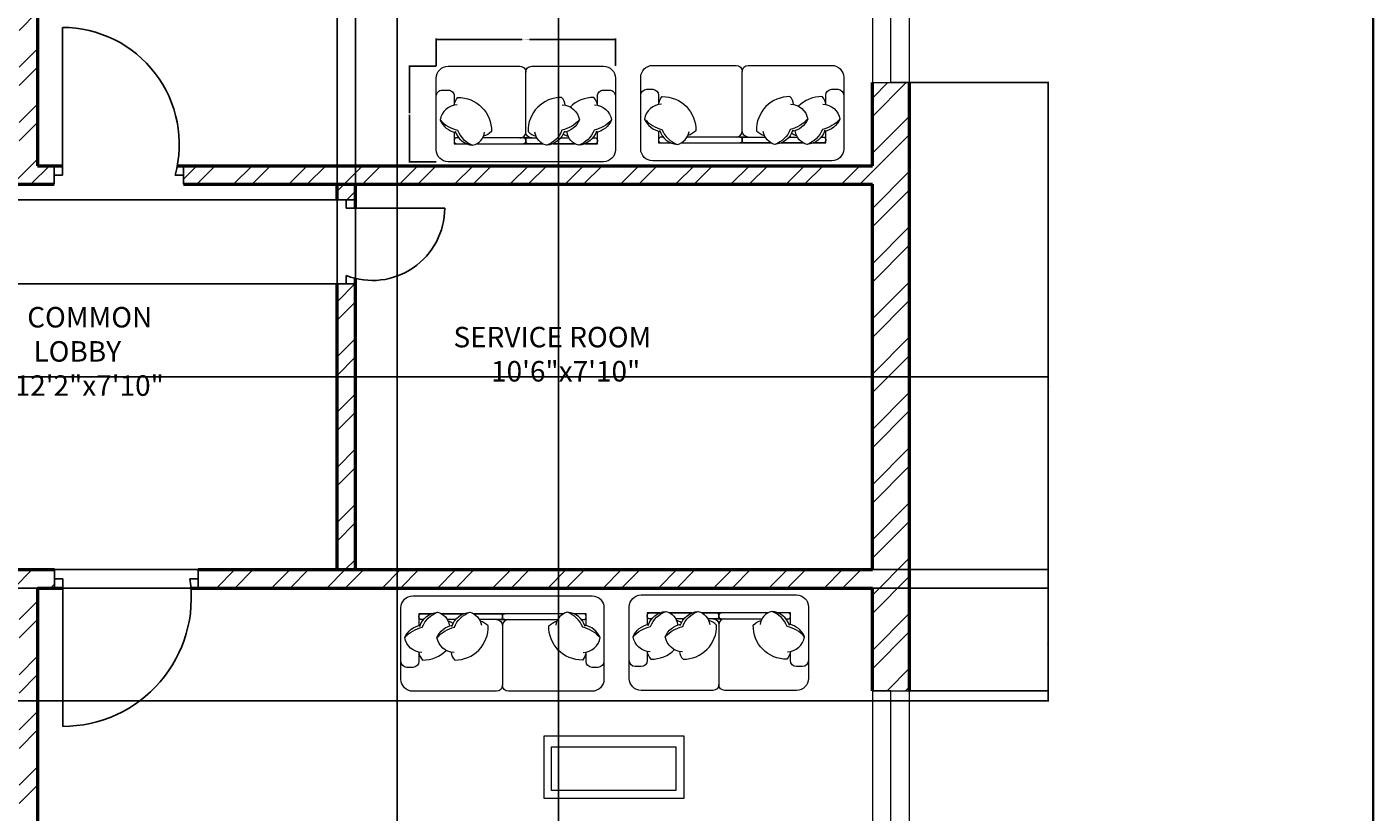
# Model space of a CAD drawing. Units: inches. Extents: x 2310 to 2937, y 1113 to 2410.
# Tile 16 of 23: x 2609 to 2937, y 1940 to 2132. Entities that reach past the tile are written whole.
import ezdxf

# ---------------------------------------------------------------- set-up
doc = ezdxf.new("R2010")
doc.units = ezdxf.units.IN
for name, color, linetype, lineweight in [('A-ANNO-DIMS', 2, 'Continuous', 18), ('A-ANNO-TTLB', 7, 'Continuous', 35), ('A-AREA-IDEN', 7, 'Continuous', 18), ('A-DOOR', 31, 'Continuous', 25), ('A-FURN', 8, 'Continuous', 18), ('A-GLAZ', 191, 'Continuous', 20), ('A-WALL', 7, 'Continuous', 50), ('A-WALL-PATT', 85, 'Continuous', 13)]:
    doc.layers.add(name, color=color, linetype=linetype, lineweight=lineweight)
doc.styles.get("Standard").update_dxf_attribs({"font": 'arial.ttf'})
doc.dimstyles.get("Standard").update_dxf_attribs({"dimtxt": 0.18, "dimasz": 0.18, "dimexe": 0.18, "dimexo": 0.0625, "dimgap": 0.09, "dimtad": 0, "dimtih": 1, "dimtoh": 1, "dimdec": 4, "dimzin": 0, "dimdsep": 46, "dimtxsty": 'Standard', "dimcen": 0.09, "dimadec": 0, "dimazin": 0, "dimtfac": 1, "dimtdec": 4, "dimtofl": 0, "dimtmove": 0, "dimatfit": 3, "dimfxl": 1, "dimtolj": 1, "dimtzin": 0, "dimarcsym": 0})

# ---------------------------------------------------------------- blocks, each defined once
blk = doc.blocks.new('SOFA-COMPACT')
at = {"ltscale": 0.03}
blk.add_lwpolyline([(20.37, 23.28, -0.414214), (21.83, 21.83, -0.414214), (23.28, 23.28), (40.75, 23.28, -0.414214), (43.66, 20.37), (43.66, 2.91, -0.414214), (40.75, 0), (2.91, 0, -0.414214), (0, 2.91), (0, 20.37, -0.414214), (2.91, 23.28), (20.37, 23.28, -0.414214), (21.83, 21.83, -0.414214), (23.28, 23.28)], format="xyb", dxfattribs=at)
for points in [[(20.37, 5.82, 0.414214), (21.83, 7.28), (21.83, 21.83, 0.414214)], [(23.28, 5.82, -0.414214), (21.83, 7.28), (21.83, 21.83, -0.414214)], [(0, 16.01, -0.414214), (1.46, 17.46), (2.91, 17.46, -0.414214), (4.37, 16.01), (4.37, 13.75)], [(39.29, 13.75), (39.29, 16.01, -0.414214), (40.75, 17.46), (42.2, 17.46, -0.414214), (43.66, 16.01)], [(5.1, 13.84, 0.356772), (0.93, 10.17, 0.249542), (4.7, 7.15, -9.61688)], [(4.36, 13.75, -0.165541), (5.26, 15.67, -0.425989), (13.44, 7.34, -0.121523), (11.5, 6.19, 7.115464)], [(31.45, 13.75, 0.165541), (30.55, 15.67, 0.425989), (22.38, 7.34, 0.121523), (24.32, 6.19, -7.115464)], [(30.72, 13.84, -0.356772), (34.89, 10.17, -0.249542), (31.11, 7.15, 9.61688)], [(39.29, 13.75, 0.165541), (38.39, 15.67, 0.200231), (32.62, 13.33, 0.121523)], [(38.56, 13.84, -0.356772), (42.73, 10.17, -0.249542), (38.95, 7.15, 9.61688)], [(0.93, 10.17, 0.14773), (5.18, 7.67, 0.213343), (8.93, 4, 0.178662)], [(34.89, 10.17, -0.14773), (30.64, 7.67, -0.213343), (26.88, 4, -0.178662)], [(42.73, 10.17, -0.14773), (38.48, 7.67, -0.213343), (34.72, 4, -0.178662)], [(4.59, 7.47, 0.306663), (8.93, 4, 0.30633), (11.77, 7.17, -0.872847)], [(20.37, 5.82, 0.414214), (21.83, 7.28)], [(23.28, 5.82, -0.414214), (21.83, 7.28)], [(31.22, 7.47, -0.306663), (26.88, 4, -0.30633), (24.05, 7.17, 0.872847)], [(30.94, 6.76, 0.071865), (32.16, 6.19, -7.115464)], [(39.06, 7.47, -0.306663), (34.72, 4, -0.30633), (31.89, 7.17, 0.872847)], [(36.23, 4.37), (39.29, 4.37), (39.29, 7.23, -0.414214)], [(5.48, 5.82), (4.95, 5.82, 0.414214), (4.37, 5.24), (4.37, 4.95, 0.414214), (4.95, 4.37)], [(4.95, 4.37), (7.43, 4.37, 0.414214)], [(9.85, 4.37), (21.25, 4.37, 0.414214), (21.83, 4.95), (21.83, 5.24, 0.414214), (21.25, 5.82), (11.31, 5.82, 0.414214)], [(25.97, 4.37), (22.41, 4.37, -0.414214), (21.83, 4.95), (21.83, 5.24, -0.414214), (22.41, 5.82), (24.5, 5.82, -0.414214)], [(33.81, 4.37), (28.39, 4.37, -0.414214)], [(30.34, 5.82), (32.34, 5.82, -0.414214)], [(38.71, 4.37), (36.23, 4.37, -0.414214)], [(38.18, 5.82), (38.71, 5.82, -0.414214), (39.29, 5.24), (39.29, 4.95, -0.414214), (38.71, 4.37)]]:
    blk.add_lwpolyline(points, format="xyb")
for points in [[(4.37, 7.23), (4.37, 4.37), (7.43, 4.37)], [(9.85, 4.37), (25.97, 4.37)], [(28.39, 4.37), (33.81, 4.37)]]:
    blk.add_lwpolyline(points)
blk.add_lwpolyline([(21.25, 4.37), (22.41, 4.37, -0.414214), (21.83, 4.95), (21.83, 5.24, -0.414214), (22.41, 5.82), (21.25, 5.82, -0.414214), (21.83, 5.24), (21.83, 4.95, -0.414214)], format="xyb", close=True)
blk = doc.blocks.new('WIN-60IN')
for p, q in [((4.5, 60), (0, 60)), ((0, 60), (9, 60)), ((0, 60), (0, 0)), ((4.5, 0), (4.5, 60)), ((9, 60), (9, 0)), ((0, 0), (9, 0)), ((9, 0), (4.5, 0))]:
    blk.add_line(p, q)
blk = doc.blocks.new('*D37')
at = {"layer": 'A-ANNO-DIMS', "color": 0, "lineweight": -2, "transparency": 16777216}
for p, q in [((2708.68, 2122.37), (2708.68, 2129.03)), ((2708.86, 2128.85), (2729.6, 2128.85)), ((2752.16, 2128.85), (2731.41, 2128.85)), ((2752.34, 2122.37), (2752.34, 2129.03))]:
    blk.add_line(p, q, dxfattribs=at)
at = {"layer": 'A-ANNO-DIMS', "color": 0, "transparency": 16777216}
for points in [[(2708.86, 2128.88), (2708.86, 2128.82), (2708.68, 2128.85)], [(2752.16, 2128.88), (2752.16, 2128.82), (2752.34, 2128.85)]]:
    blk.add_solid(points, dxfattribs=at)
at = {"layer": 'Defpoints', "color": 0, "transparency": 16777216}
for p in [(2752.34, 2128.85), (2708.68, 2122.3), (2752.34, 2122.3)]:
    blk.add_point(p, dxfattribs=at)
at = {"layer": 'A-ANNO-DIMS', "color": 0, "transparency": 16777216, "insert": (2730.51, 2128.85), "char_height": 0.18, "attachment_point": 5}
blk.add_mtext('\\A1;SOFA 44 TYP.', dxfattribs=at)
blk = doc.blocks.new('*D38')
at = {"layer": 'A-ANNO-DIMS', "color": 0, "lineweight": -2, "transparency": 16777216}
for p, q in [((2708.62, 2122.3), (2701.95, 2122.3)), ((2702.13, 2122.12), (2702.13, 2110.84)), ((2702.13, 2099.2), (2702.13, 2110.48)), ((2708.62, 2099.02), (2701.95, 2099.02))]:
    blk.add_line(p, q, dxfattribs=at)
at = {"layer": 'A-ANNO-DIMS', "color": 0, "transparency": 16777216}
for points in [[(2702.1, 2122.12), (2702.16, 2122.12), (2702.13, 2122.3)], [(2702.1, 2099.2), (2702.16, 2099.2), (2702.13, 2099.02)]]:
    blk.add_solid(points, dxfattribs=at)
at = {"layer": 'Defpoints', "color": 0, "transparency": 16777216}
for p in [(2702.13, 2122.3), (2708.68, 2122.3), (2708.68, 2099.02)]:
    blk.add_point(p, dxfattribs=at)
at = {"layer": 'A-ANNO-DIMS', "color": 0, "transparency": 16777216, "insert": (2702.13, 2110.66), "char_height": 0.18, "attachment_point": 5}
blk.add_mtext('\\A1;23 TYP.', dxfattribs=at)
blk = doc.blocks.new('*D42')
at = {"layer": 'A-ANNO-DIMS', "color": 0, "lineweight": -2, "transparency": 16777216}
for p, q in [((2699.14, 2347.45), (2699.14, 1649.5)), ((2738.49, 2347.45), (2738.49, 1649.5)), ((2699.32, 1649.68), (2718.42, 1649.68)), ((2738.31, 1649.68), (2719.21, 1649.68))]:
    blk.add_line(p, q, dxfattribs=at)
at = {"layer": 'A-ANNO-DIMS', "color": 0, "transparency": 16777216}
for points in [[(2699.32, 1649.71), (2699.32, 1649.65), (2699.14, 1649.68)], [(2738.31, 1649.71), (2738.31, 1649.65), (2738.49, 1649.68)]]:
    blk.add_solid(points, dxfattribs=at)
at = {"layer": 'Defpoints', "color": 0, "transparency": 16777216}
for p in [(2699.14, 2347.51), (2738.49, 2347.51), (2738.49, 1649.68)]:
    blk.add_point(p, dxfattribs=at)
at = {"layer": 'A-ANNO-DIMS', "color": 0, "transparency": 16777216, "insert": (2718.81, 1649.68), "char_height": 0.18, "attachment_point": 5}
blk.add_mtext('\\A1;39.35', dxfattribs=at)
blk = doc.blocks.new('*D48')
at = {"layer": 'A-ANNO-DIMS', "color": 0, "lineweight": -2, "transparency": 16777216}
for p, q in [((2824.05, 2118.3), (2858.02, 2118.3)), ((2857.84, 2118.12), (2857.84, 2044.32)), ((2857.84, 1970.16), (2857.84, 2043.96)), ((2824.05, 1969.98), (2858.02, 1969.98))]:
    blk.add_line(p, q, dxfattribs=at)
at = {"layer": 'A-ANNO-DIMS', "color": 0, "transparency": 16777216}
for points in [[(2857.81, 2118.12), (2857.87, 2118.12), (2857.84, 2118.3)], [(2857.81, 1970.16), (2857.87, 1970.16), (2857.84, 1969.98)]]:
    blk.add_solid(points, dxfattribs=at)
at = {"layer": 'Defpoints', "color": 0, "transparency": 16777216}
for p in [(2823.99, 2118.3), (2857.84, 2118.3), (2823.99, 1969.98)]:
    blk.add_point(p, dxfattribs=at)
at = {"layer": 'A-ANNO-DIMS', "color": 0, "transparency": 16777216, "insert": (2857.84, 2044.14), "char_height": 0.18, "attachment_point": 5}
blk.add_mtext('\\A1;148.32', dxfattribs=at)
blk = doc.blocks.new('*D57')
at = {"layer": 'A-ANNO-DIMS', "color": 0, "lineweight": -2, "transparency": 16777216}
for p, q in [((2403.55, 1995.01), (2858.02, 1995.01)), ((2857.84, 1994.83), (2857.84, 1981.45)), ((2857.84, 1967.7), (2857.84, 1981.09)), ((2403.55, 1967.52), (2858.02, 1967.52))]:
    blk.add_line(p, q, dxfattribs=at)
at = {"layer": 'A-ANNO-DIMS', "color": 0, "transparency": 16777216}
for points in [[(2857.81, 1994.83), (2857.87, 1994.83), (2857.84, 1995.01)], [(2857.81, 1967.7), (2857.87, 1967.7), (2857.84, 1967.52)]]:
    blk.add_solid(points, dxfattribs=at)
at = {"layer": 'Defpoints', "color": 0, "transparency": 16777216}
for p in [(2403.49, 1995.01), (2403.49, 1967.52), (2857.84, 1967.52)]:
    blk.add_point(p, dxfattribs=at)
at = {"layer": 'A-ANNO-DIMS', "color": 0, "transparency": 16777216, "insert": (2857.84, 1981.27), "char_height": 0.18, "attachment_point": 5}
blk.add_mtext('\\A1;27.49', dxfattribs=at)
blk = doc.blocks.new('*D64')
at = {"layer": 'A-ANNO-DIMS', "color": 0, "lineweight": -2, "transparency": 16777216}
for p, q in [((2524.527191, 2046.513944), (2858.015941, 2046.513944)), ((2857.835941, 2046.333944), (2857.835941, 2023.193944)), ((2857.835941, 1999.693944), (2857.835941, 2022.833944)), ((2524.527191, 1999.513944), (2858.015941, 1999.513944))]:
    blk.add_line(p, q, dxfattribs=at)
at = {"layer": 'A-ANNO-DIMS', "color": 0, "transparency": 16777216}
for points in [[(2857.805941, 2046.333944), (2857.865941, 2046.333944), (2857.835941, 2046.513944)], [(2857.805941, 1999.693944), (2857.865941, 1999.693944), (2857.835941, 1999.513944)]]:
    blk.add_solid(points, dxfattribs=at)
at = {"layer": 'Defpoints', "color": 0, "transparency": 16777216}
for p in [(2524.464691, 2046.513944), (2857.835941, 2046.513944), (2524.464691, 1999.513944)]:
    blk.add_point(p, dxfattribs=at)
at = {"layer": 'A-ANNO-DIMS', "color": 0, "transparency": 16777216, "insert": (2857.835941, 2023.013944), "char_height": 0.18, "attachment_point": 5}
blk.add_mtext('\\A1;47', dxfattribs=at)
blk = doc.blocks.new('*D67')
at = {"layer": 'A-ANNO-DIMS', "color": 0, "lineweight": -2, "transparency": 16777216}
for p, q in [((2684.42, 2089.69), (2360.46, 2089.69)), ((2360.64, 2089.51), (2360.64, 2079.64)), ((2360.64, 2069.41), (2360.64, 2079.28)), ((2684.42, 2069.23), (2360.46, 2069.23))]:
    blk.add_line(p, q, dxfattribs=at)
at = {"layer": 'A-ANNO-DIMS', "color": 0, "transparency": 16777216}
for points in [[(2360.61, 2089.51), (2360.67, 2089.51), (2360.64, 2089.69)], [(2360.61, 2069.41), (2360.67, 2069.41), (2360.64, 2069.23)]]:
    blk.add_solid(points, dxfattribs=at)
at = {"layer": 'Defpoints', "color": 0, "transparency": 16777216}
for p in [(2360.64, 2089.69), (2684.49, 2089.69), (2684.49, 2069.23)]:
    blk.add_point(p, dxfattribs=at)
at = {"layer": 'A-ANNO-DIMS', "color": 0, "transparency": 16777216, "insert": (2360.64, 2079.46), "char_height": 0.18, "attachment_point": 5}
blk.add_mtext('\\A1;20.46', dxfattribs=at)
blk = doc.blocks.new('*D68')
at = {"layer": 'A-ANNO-DIMS', "color": 0, "lineweight": -2, "transparency": 16777216}
for p, q in [((2684.49, 1999.58), (2684.49, 2390.54)), ((2684.67, 2390.36), (2686.48, 2390.36)), ((2688.81, 2390.36), (2686.99, 2390.36)), ((2688.99, 1999.58), (2688.99, 2390.54))]:
    blk.add_line(p, q, dxfattribs=at)
at = {"layer": 'A-ANNO-DIMS', "color": 0, "transparency": 16777216}
for points in [[(2684.67, 2390.39), (2684.67, 2390.33), (2684.49, 2390.36)], [(2688.81, 2390.39), (2688.81, 2390.33), (2688.99, 2390.36)]]:
    blk.add_solid(points, dxfattribs=at)
at = {"layer": 'Defpoints', "color": 0, "transparency": 16777216}
for p in [(2688.99, 2390.36), (2684.49, 1999.51), (2688.99, 1999.51)]:
    blk.add_point(p, dxfattribs=at)
at = {"layer": 'A-ANNO-DIMS', "color": 0, "transparency": 16777216, "insert": (2686.74, 2390.36), "char_height": 0.18, "attachment_point": 5}
blk.add_mtext('\\A1;4.5', dxfattribs=at)

msp = doc.modelspace()

# ---------------------------------------------------------------- hatches: boundary and pattern name
at = {"layer": 'A-WALL-PATT'}
h = msp.add_hatch(dxfattribs=at)
h.set_pattern_fill('ANSI32', color=256)
h.paths.add_polyline_path([(2639.1394, 2356.5139), (2563.662, 2356.5139), (2563.662, 2347.5139), (2606.9859, 2347.5139), (2606.9859, 2210.5139), (2514.2692, 2210.5139), (2514.2692, 2206.0139), (2606.9859, 2206.0139), (2606.9859, 2098.0139), (2602.689, 2098.0139), (2602.689, 2093.5139), (2615.5262, 2093.5139), (2615.5262, 2095.7639), (2615.5262, 2098.0139), (2611.4859, 2098.0139), (2611.4859, 2206.0139), (2703.9391, 2206.0139), (2703.9391, 2208.2639), (2703.9391, 2210.5139), (2611.4859, 2210.5139), (2611.4859, 2347.5139), (2639.1394, 2347.5139)])
h.paths.add_polyline_path([(2823.9859, 2356.5139), (2699.1394, 2356.5139), (2699.1394, 2347.5139), (2738.4859, 2347.5139), (2738.4859, 2343.9266), (2742.9859, 2343.9266), (2742.9859, 2347.5139), (2814.9859, 2347.5139), (2814.9859, 2336.76), (2823.9859, 2336.76)])
h.paths.add_polyline_path([(2823.9859, 2312.76), (2814.9859, 2312.76), (2814.9859, 2299.5139), (2742.9859, 2299.5139), (2742.9859, 2323.0159), (2740.7359, 2323.0159), (2738.4859, 2323.0159), (2738.4859, 2210.5139), (2734.5483, 2210.5139), (2734.5483, 2206.0139), (2746.8769, 2206.0139), (2746.8769, 2208.2639), (2746.8769, 2210.5139), (2742.9859, 2210.5139), (2742.9859, 2295.0139), (2814.9859, 2295.0139), (2814.9859, 2269.8977), (2823.9859, 2269.8977)])
h.paths.add_polyline_path([(2823.9859, 2210.5139), (2823.9859, 2233.8977), (2819.4859, 2233.8977), (2814.9859, 2233.8977), (2814.9859, 2210.5139), (2769.9745, 2210.5139), (2769.9745, 2206.0139), (2814.9859, 2206.0139), (2814.9859, 2178.3027), (2823.9859, 2178.3027)])
h.paths.add_polyline_path([(2823.9859, 2118.3027), (2819.4859, 2118.3027), (2814.9859, 2118.3027), (2814.9859, 2098.0139), (2647.0333, 2098.0139), (2647.0333, 2093.5139), (2814.9859, 2093.5139), (2814.9859, 1999.5139), (2650.6052, 1999.5139), (2650.6052, 1995.0139), (2814.9859, 1995.0139), (2814.9859, 1969.9784), (2823.9859, 1969.9784)])
h.paths.add_polyline_path([(2403.4859, 2093.5139), (2569.9888, 2093.5139), (2569.9888, 2095.7639), (2569.9888, 2098.0139), (2403.4859, 2098.0139), (2403.4859, 2131.7587), (2394.4859, 2131.7587), (2394.4859, 1967.522), (2403.4859, 1967.522), (2403.4859, 1995.0139), (2569.8903, 1995.0139), (2569.8903, 1997.2639), (2569.8903, 1999.5139), (2403.4859, 1999.5139)])
h.paths.add_polyline_path([(2503.662, 2356.5139), (2394.4859, 2356.5139), (2394.4859, 2337.9231), (2398.9859, 2337.9231), (2403.4859, 2337.9231), (2403.4859, 2347.5139), (2475.4859, 2347.5139), (2475.4859, 2343.0384), (2479.9859, 2343.0384), (2479.9859, 2347.5139), (2503.662, 2347.5139)])
h.paths.add_polyline_path([(2498.3065, 1745.5139), (2479.9859, 1745.5139), (2479.9859, 1749.1663), (2477.7359, 1749.1663), (2475.4859, 1749.1663), (2475.4859, 1745.5139), (2403.4859, 1745.5139), (2403.4859, 1753.6409), (2398.9859, 1753.6409), (2394.4859, 1753.6409), (2394.4859, 1736.5139), (2498.3065, 1736.5139), (2498.3065, 1741.0139)])
h.paths.add_polyline_path([(2479.9859, 1882.5139), (2483.9367, 1882.5139), (2483.9367, 1887.0139), (2471.5501, 1887.0139), (2471.5501, 1885.1969), (2471.5501, 1882.5139), (2475.4859, 1882.5139), (2475.4859, 1798.0139), (2403.4859, 1798.0139), (2403.4859, 1828.0433), (2402.2852, 1828.0433), (2394.4859, 1828.0433), (2394.4859, 1777.6409), (2403.4859, 1777.6409), (2403.4859, 1793.5139), (2475.4859, 1793.5139), (2475.4859, 1769.1696), (2479.9859, 1769.1696)])
h.paths.add_polyline_path([(2403.4859, 1907.522), (2398.9859, 1907.522), (2394.4859, 1907.522), (2394.4859, 1864.0433), (2403.4859, 1864.0433), (2403.4859, 1882.5139), (2448.9325, 1882.5139), (2448.9325, 1884.7639), (2448.9325, 1887.0139), (2403.4859, 1887.0139)])
h.paths.add_polyline_path([(2702.2061, 1887.0139), (2611.4859, 1887.0139), (2611.4859, 1995.0139), (2615.6132, 1995.0139), (2615.6132, 1999.5139), (2602.4798, 1999.5139), (2602.4798, 1997.2639), (2602.4798, 1995.0139), (2606.9859, 1995.0139), (2606.9859, 1887.0139), (2516.2443, 1887.0139), (2516.2443, 1884.7639), (2516.2443, 1882.5139), (2606.9859, 1882.5139), (2606.9859, 1745.5139), (2558.3065, 1745.5139), (2558.3065, 1736.5139), (2638.8921, 1736.5139), (2638.8921, 1741.0139), (2638.8921, 1745.5139), (2611.4859, 1745.5139), (2611.4859, 1882.5139), (2702.2061, 1882.5139)])
h.paths.add_polyline_path([(2823.9859, 1909.9784), (2819.4859, 1909.9784), (2814.9859, 1909.9784), (2814.9859, 1887.0139), (2769.144, 1887.0139), (2769.144, 1884.7639), (2769.144, 1882.5139), (2814.9859, 1882.5139), (2814.9859, 1854.1704), (2823.9859, 1854.1704)])
h.paths.add_polyline_path([(2823.9859, 1818.1704), (2819.4859, 1818.1704), (2814.9859, 1818.1704), (2814.9859, 1798.0139), (2742.9859, 1798.0139), (2742.9859, 1882.5139), (2746.805, 1882.5139), (2746.805, 1887.0139), (2733.7334, 1887.0139), (2733.7334, 1884.7639), (2733.7334, 1882.5139), (2738.4859, 1882.5139), (2738.4859, 1771.1728), (2740.7359, 1771.1728), (2742.9859, 1771.1728), (2742.9859, 1793.5139), (2814.9859, 1793.5139), (2814.9859, 1783.6684), (2823.9859, 1783.6684)])
h.paths.add_polyline_path([(2823.9859, 1759.6684), (2814.9859, 1759.6684), (2814.9859, 1745.5139), (2742.9859, 1745.5139), (2742.9859, 1748.9831), (2740.7359, 1748.9831), (2738.4859, 1748.9831), (2738.4859, 1745.5139), (2698.8921, 1745.5139), (2698.8921, 1736.5139), (2823.9859, 1736.5139)])
h = msp.add_hatch(dxfattribs=at)
h.set_pattern_fill('ANSI32', color=256)
h.paths.add_polyline_path([(2688.9859, 2069.228), (2686.7359, 2069.228), (2684.4859, 2069.228), (2684.4859, 1999.5139), (2688.9859, 1999.5139)])
h.paths.add_polyline_path([(2688.9859, 2093.5139), (2684.4859, 2093.5139), (2684.4859, 2089.6861), (2688.9859, 2089.6861)])

# ---------------------------------------------------------------- linework, layer by layer
at = {"layer": 'A-ANNO-TTLB'}
msp.add_lwpolyline([(2310.2498, 2409.8427), (2937.0534, 2409.8427), (2937.0534, 1616.036), (2310.2498, 1616.036)], close=True, dxfattribs=at)
at = {"layer": 'A-DOOR'}
for p, q in [((2617.5262, 2095.7639), (2617.5262, 2131.7639)), ((2615.5262, 2098.0139), (2615.5262, 2093.5139)), ((2647.0333, 2098.0139), (2647.0333, 2093.5139)), ((2615.5262, 2093.5139), (2615.5262, 2095.7639)), ((2615.5262, 2095.7639), (2617.5262, 2095.7639)), ((2647.0333, 2095.7639), (2645.0333, 2095.7639)), ((2647.0333, 2093.5139), (2647.0333, 2095.7639)), ((2684.4859, 2089.6861), (2688.9859, 2089.6861)), ((2688.9859, 2089.6861), (2686.7359, 2089.6861)), ((2686.7359, 2089.6861), (2686.7359, 2087.6861)), ((2686.7359, 2087.6861), (2710.7359, 2087.6861)), ((2686.7359, 2069.228), (2686.7359, 2071.228)), ((2684.4859, 2069.228), (2688.9859, 2069.228)), ((2688.9859, 2069.228), (2686.7359, 2069.228)), ((2615.6132, 1995.0139), (2615.6132, 1999.5139)), ((2615.6132, 1999.5139), (2615.6132, 1997.2639)), ((2650.6052, 1999.5139), (2650.6052, 1999.5139)), ((2650.6052, 1999.5139), (2650.6052, 1995.0139)), ((2615.6132, 1997.2639), (2617.6132, 1997.2639)), ((2617.6132, 1997.2639), (2617.6132, 1961.2639)), ((2650.6052, 1997.2639), (2648.6052, 1997.2639)), ((2650.6052, 1995.0139), (2650.6052, 1997.2639)), ((2650.6052, 1997.2639), (2650.6052, 1997.2639))]:
    msp.add_line(p, q, dxfattribs=at)
for centre, radius, start, end in [((2617.5262, 2103.2551), 28.5089, 344.765874, 90), ((2693.0928, 2087.6861), 17.6431, 248.881039, 0), ((2617.6132, 1992.6044), 31.3404, 270, 8.550242)]:
    msp.add_arc(centre, radius, start, end, dxfattribs=at)
at = {"layer": 'A-FURN', "ltscale": 0.03}
for points in [[(2781.8049, 2122.4997, -0.41421356), (2783.26, 2121.0445, -0.41421356), (2784.7152, 2122.4997), (2805.0879, 2122.4997, -0.41421356), (2807.9983, 2119.5893), (2807.9983, 2102.1271, -0.41421356), (2805.0879, 2099.2167), (2761.4322, 2099.2167, -0.41421356), (2758.5218, 2102.1271), (2758.5218, 2119.5893, -0.41421356), (2761.4322, 2122.4997), (2781.8049, 2122.4997, -0.41421356), (2783.26, 2121.0445, -0.41421356), (2784.7152, 2122.4997)], [(2726.2708, 1969.8431, -0.41421356), (2724.8156, 1971.2983, -0.41421356), (2723.3604, 1969.8431), (2702.9878, 1969.8431, -0.41421356), (2700.0774, 1972.7535), (2700.0774, 1990.2158, -0.41421356), (2702.9878, 1993.1262), (2746.6434, 1993.1262, -0.41421356), (2749.5538, 1990.2158), (2749.5538, 1972.7535, -0.41421356), (2746.6434, 1969.8431), (2726.2708, 1969.8431, -0.41421356), (2724.8156, 1971.2983, -0.41421356), (2723.3604, 1969.8431)], [(2779.0221, 1970.0386, -0.41421356), (2777.5669, 1971.4938, -0.41421356), (2776.1118, 1970.0386), (2758.6495, 1970.0386, -0.41421356), (2755.7391, 1972.949), (2755.7391, 1990.4113, -0.41421356), (2758.6495, 1993.3217), (2796.4844, 1993.3217, -0.41421356), (2799.3948, 1990.4113), (2799.3948, 1972.949, -0.41421356), (2796.4844, 1970.0386), (2779.0221, 1970.0386, -0.41421356), (2777.5669, 1971.4938, -0.41421356), (2776.1118, 1970.0386)]]:
    msp.add_lwpolyline(points, format="xyb", dxfattribs=at)
at = {"layer": 'A-FURN'}
for points in [[(2781.8049, 2105.0374, 0.41421356), (2783.26, 2106.4926), (2783.26, 2121.0445, 0.41421356)], [(2784.7152, 2105.0374, -0.41421356), (2783.26, 2106.4926), (2783.26, 2121.0445, -0.41421356)], [(2758.5218, 2115.2238, -0.41421356), (2759.977, 2116.679), (2761.4322, 2116.679, -0.41421356), (2762.8874, 2115.2238), (2762.8874, 2112.9691)], [(2803.6327, 2112.9691), (2803.6327, 2115.2238, -0.41421356), (2805.0879, 2116.679), (2806.5431, 2116.679, -0.41421356), (2807.9983, 2115.2238)], [(2762.8842, 2112.9685, -0.16554063), (2763.7845, 2114.8912, -0.42598917), (2771.9571, 2106.5549, -0.12152332), (2770.0171, 2105.4059, 7.11546429)], [(2795.7968, 2112.9685, 0.16554063), (2794.8966, 2114.8912, 0.42598917), (2786.724, 2106.5549, 0.12152332), (2788.664, 2105.4059, -7.11546429)], [(2803.6359, 2112.9685, 0.16554063), (2802.7356, 2114.8912, 0.20023115), (2796.9591, 2112.5495, 0.12152332)], [(2763.6177, 2113.0572, 0.35677236), (2759.448, 2109.3892, 0.24954205), (2763.2261, 2106.3665, -9.61688035)], [(2795.0634, 2113.0572, -0.35677236), (2799.2331, 2109.3892, -0.24954205), (2795.4549, 2106.3665, 9.61688035)], [(2802.9024, 2113.0572, -0.35677236), (2807.0721, 2109.3892, -0.24954205), (2803.294, 2106.3665, 9.61688035)], [(2759.448, 2109.3892, 0.14772988), (2763.7011, 2106.8884, 0.21334276), (2767.4538, 2103.2204, 0.17866181)], [(2799.2331, 2109.3892, -0.14772988), (2794.98, 2106.8884, -0.21334276), (2791.2272, 2103.2204, -0.17866181)], [(2807.0721, 2109.3892, -0.14772988), (2802.819, 2106.8884, -0.21334276), (2799.0663, 2103.2204, -0.17866181)], [(2763.9979, 2105.0374), (2763.4695, 2105.0374, 0.41421356), (2762.8874, 2104.4554), (2762.8874, 2104.1643, 0.41421356), (2763.4695, 2103.5823)], [(2763.1135, 2106.689, 0.30666349), (2767.4538, 2103.2204, 0.30632997), (2770.2892, 2106.3882, -0.87284716)], [(2763.4695, 2103.5823), (2765.9487, 2103.5823, 0.41421356)], [(2768.3696, 2103.5823), (2782.678, 2103.5823, 0.41421356), (2783.26, 2104.1643), (2783.26, 2104.4554, 0.41421356), (2782.678, 2105.0374), (2769.8349, 2105.0374, 0.41421356)], [(2781.8049, 2105.0374, 0.41421356), (2783.26, 2106.4926)], [(2784.7152, 2105.0374, -0.41421356), (2783.26, 2106.4926)], [(2790.3114, 2103.5823), (2783.8421, 2103.5823, -0.41421356), (2783.26, 2104.1643), (2783.26, 2104.4554, -0.41421356), (2783.8421, 2105.0374), (2788.8461, 2105.0374, -0.41421356)], [(2795.5675, 2106.689, -0.30666349), (2791.2272, 2103.2204, -0.30632997), (2788.3918, 2106.3882, 0.87284716)], [(2798.1505, 2103.5823), (2792.7323, 2103.5823, -0.41421356)], [(2794.6832, 2105.0374), (2796.6852, 2105.0374, -0.41421356)], [(2795.283, 2105.9748, 0.07186538), (2796.503, 2105.4059, -7.11546429)], [(2803.4066, 2106.689, -0.30666349), (2799.0663, 2103.2204, -0.30632997), (2796.2309, 2106.3882, 0.87284716)], [(2800.5714, 2103.5823), (2803.6327, 2103.5823), (2803.6327, 2106.442, -0.41421356)], [(2803.0506, 2103.5823), (2800.5714, 2103.5823, -0.41421356)], [(2802.5222, 2105.0374), (2803.0506, 2105.0374, -0.41421356), (2803.6327, 2104.4554), (2803.6327, 2104.1643, -0.41421356), (2803.0506, 2103.5823)], [(2701.0035, 1982.9536, -0.14772988), (2705.2566, 1985.4545, -0.21334276), (2709.0094, 1989.1225, -0.17866181)], [(2707.5043, 1988.7606), (2704.443, 1988.7606), (2704.443, 1985.9008, -0.41421356)], [(2705.5534, 1987.3054), (2705.025, 1987.3054, -0.41421356), (2704.443, 1987.8875), (2704.443, 1988.1785, -0.41421356), (2705.025, 1988.7606)], [(2704.6691, 1985.6538, -0.30666349), (2709.0094, 1989.1225, -0.30632997), (2711.8448, 1985.9547, 0.87284716)], [(2705.025, 1988.7606), (2707.5043, 1988.7606, -0.41421356)], [(2708.8426, 1982.9536, -0.14772988), (2713.0957, 1985.4545, -0.21334276), (2716.8484, 1989.1225, -0.17866181)], [(2709.9252, 1988.7606), (2715.3433, 1988.7606, -0.41421356)], [(2712.5081, 1985.6538, -0.30666349), (2716.8484, 1989.1225, -0.30632997), (2719.6838, 1985.9547, 0.87284716)], [(2717.7642, 1988.7606), (2724.2335, 1988.7606, -0.41421356), (2724.8156, 1988.1785), (2724.8156, 1987.8875, -0.41421356), (2724.2335, 1987.3054), (2719.2295, 1987.3054, -0.41421356)], [(2739.706, 1988.7606), (2725.3977, 1988.7606, 0.41421356), (2724.8156, 1988.1785), (2724.8156, 1987.8875, 0.41421356), (2725.3977, 1987.3054), (2738.2407, 1987.3054, 0.41421356)], [(2744.9622, 1985.6538, 0.30666349), (2740.6218, 1989.1225, 0.30632997), (2737.7864, 1985.9547, -0.87284716)], [(2748.6277, 1982.9536, 0.14772988), (2744.3746, 1985.4545, 0.21334276), (2740.6218, 1989.1225, 0.17866181)], [(2744.6062, 1988.7606), (2742.1269, 1988.7606, 0.41421356)], [(2744.0778, 1987.3054), (2744.6062, 1987.3054, 0.41421356), (2745.1882, 1987.8875), (2745.1882, 1988.1785, 0.41421356), (2744.6062, 1988.7606)], [(2756.6652, 1983.1491, -0.14772988), (2760.9183, 1985.65, -0.21334276), (2764.6711, 1989.318, -0.17866181)], [(2763.166, 1988.9561), (2760.1047, 1988.9561), (2760.1047, 1986.0963, -0.41421356)], [(2761.2152, 1987.5009), (2760.6868, 1987.5009, -0.41421356), (2760.1047, 1988.083), (2760.1047, 1988.374, -0.41421356), (2760.6868, 1988.9561)], [(2760.3308, 1985.8493, -0.30666349), (2764.6711, 1989.318, -0.30632997), (2767.5065, 1986.1502, 0.87284716)], [(2760.6868, 1988.9561), (2763.166, 1988.9561, -0.41421356)], [(2764.5043, 1983.1491, -0.14772988), (2768.7574, 1985.65, -0.21334276), (2772.5101, 1989.318, -0.17866181)], [(2765.5869, 1988.9561), (2771.005, 1988.9561, -0.41421356)], [(2768.1698, 1985.8493, -0.30666349), (2772.5101, 1989.318, -0.30632997), (2775.3455, 1986.1502, 0.87284716)], [(2773.4259, 1988.9561), (2776.9849, 1988.9561, -0.41421356), (2777.5669, 1988.374), (2777.5669, 1988.083, -0.41421356), (2776.9849, 1987.5009), (2774.8912, 1987.5009, -0.41421356)], [(2789.547, 1988.9561), (2778.149, 1988.9561, 0.41421356), (2777.5669, 1988.374), (2777.5669, 1988.083, 0.41421356), (2778.149, 1987.5009), (2788.0817, 1987.5009, 0.41421356)], [(2794.8031, 1985.8493, 0.30666349), (2790.4628, 1989.318, 0.30632997), (2787.6274, 1986.1502, -0.87284716)], [(2798.4686, 1983.1491, 0.14772988), (2794.2155, 1985.65, 0.21334276), (2790.4628, 1989.318, 0.17866181)], [(2794.4471, 1988.9561), (2791.9679, 1988.9561, 0.41421356)], [(2793.9187, 1987.5009), (2794.4471, 1987.5009, 0.41421356), (2795.0292, 1988.083), (2795.0292, 1988.374, 0.41421356), (2794.4471, 1988.9561)], [(2705.1732, 1979.2856, -0.35677236), (2701.0035, 1982.9536, -0.24954205), (2704.7817, 1985.9763, 9.61688035)], [(2713.0123, 1979.2856, -0.35677236), (2708.8426, 1982.9536, -0.24954205), (2712.6207, 1985.9763, 9.61688035)], [(2713.3925, 1987.3054), (2711.3905, 1987.3054, -0.41421356)], [(2712.7926, 1986.368, 0.07186538), (2711.5726, 1986.937, -7.11546429)], [(2712.2788, 1979.3744, 0.16554063), (2713.1791, 1977.4516, 0.42598917), (2721.3517, 1985.7879, 0.12152332), (2719.4117, 1986.937, -7.11546429)], [(2723.3604, 1987.3054, -0.41421356), (2724.8156, 1985.8502)], [(2723.3604, 1987.3054, -0.41421356), (2724.8156, 1985.8502), (2724.8156, 1971.2983, -0.41421356)], [(2726.2708, 1987.3054, 0.41421356), (2724.8156, 1985.8502)], [(2726.2708, 1987.3054, 0.41421356), (2724.8156, 1985.8502), (2724.8156, 1971.2983, 0.41421356)], [(2745.1914, 1979.3744, -0.16554063), (2744.2912, 1977.4516, -0.42598917), (2736.1186, 1985.7879, -0.12152332), (2738.0586, 1986.937, 7.11546429)], [(2744.458, 1979.2856, 0.35677236), (2748.6277, 1982.9536, 0.24954205), (2744.8495, 1985.9763, -9.61688035)], [(2760.835, 1979.4811, -0.35677236), (2756.6652, 1983.1491, -0.24954205), (2760.4434, 1986.1718, 9.61688035)], [(2768.674, 1979.4811, -0.35677236), (2764.5043, 1983.1491, -0.24954205), (2768.2824, 1986.1718, 9.61688035)], [(2769.0542, 1987.5009), (2767.0522, 1987.5009, -0.41421356)], [(2768.4543, 1986.5635, 0.07186538), (2767.2343, 1987.1325, -7.11546429)], [(2767.9406, 1979.5699, 0.16554063), (2768.8408, 1977.6471, 0.42598917), (2777.0134, 1985.9834, 0.12152332), (2775.0734, 1987.1325, -7.11546429)], [(2776.1118, 1987.5009, -0.41421356), (2777.5669, 1986.0457)], [(2776.1118, 1987.5009, -0.41421356), (2777.5669, 1986.0457), (2777.5669, 1971.4938, -0.41421356)], [(2779.0221, 1987.5009, 0.41421356), (2777.5669, 1986.0457)], [(2779.0221, 1987.5009, 0.41421356), (2777.5669, 1986.0457), (2777.5669, 1971.4938, 0.41421356)], [(2795.0324, 1979.5699, -0.16554063), (2794.1322, 1977.6471, -0.42598917), (2785.9595, 1985.9834, -0.12152332), (2787.8996, 1987.1325, 7.11546429)], [(2794.2989, 1979.4811, 0.35677236), (2798.4686, 1983.1491, 0.24954205), (2794.6905, 1986.1718, -9.61688035)], [(2704.443, 1979.3737), (2704.443, 1977.1191, -0.41421356), (2702.9878, 1975.6639), (2701.5326, 1975.6639, -0.41421356), (2700.0774, 1977.1191)], [(2704.4398, 1979.3744, 0.16554063), (2705.34, 1977.4516, 0.20023115), (2711.1166, 1979.7933, 0.12152332)], [(2749.5538, 1977.1191, -0.41421356), (2748.0986, 1975.6639), (2746.6434, 1975.6639, -0.41421356), (2745.1882, 1977.1191), (2745.1882, 1979.3737)], [(2760.1047, 1979.5692), (2760.1047, 1977.3146, -0.41421356), (2758.6495, 1975.8594), (2757.1943, 1975.8594, -0.41421356), (2755.7391, 1977.3146)], [(2760.1015, 1979.5699, 0.16554063), (2761.0017, 1977.6471, 0.20023115), (2766.7783, 1979.9888, 0.12152332)], [(2799.3948, 1977.3146, -0.41421356), (2797.9396, 1975.8594), (2796.4844, 1975.8594, -0.41421356), (2795.0292, 1977.3146), (2795.0292, 1979.5692)]]:
    msp.add_lwpolyline(points, format="xyb", dxfattribs=at)
for points in [[(2762.8874, 2106.442), (2762.8874, 2103.5823), (2765.9487, 2103.5823)], [(2768.3696, 2103.5823), (2790.3114, 2103.5823)], [(2792.7323, 2103.5823), (2798.1505, 2103.5823)], [(2715.3433, 1988.7606), (2709.9252, 1988.7606)], [(2739.706, 1988.7606), (2717.7642, 1988.7606)], [(2745.1882, 1985.9008), (2745.1882, 1988.7606), (2742.1269, 1988.7606)], [(2771.005, 1988.9561), (2765.5869, 1988.9561)], [(2789.547, 1988.9561), (2773.4259, 1988.9561)], [(2795.0292, 1986.0963), (2795.0292, 1988.9561), (2791.9679, 1988.9561)]]:
    msp.add_lwpolyline(points, dxfattribs=at)
for points in [[(2782.678, 2103.5823), (2783.8421, 2103.5823, -0.41421356), (2783.26, 2104.1643), (2783.26, 2104.4554, -0.41421356), (2783.8421, 2105.0374), (2782.678, 2105.0374, -0.41421356), (2783.26, 2104.4554), (2783.26, 2104.1643, -0.41421356)], [(2725.3977, 1988.7606), (2724.2335, 1988.7606, -0.41421356), (2724.8156, 1988.1785), (2724.8156, 1987.8875, -0.41421356), (2724.2335, 1987.3054), (2725.3977, 1987.3054, -0.41421356), (2724.8156, 1987.8875), (2724.8156, 1988.1785, -0.41421356)], [(2778.149, 1988.9561), (2776.9849, 1988.9561, -0.41421356), (2777.5669, 1988.374), (2777.5669, 1988.083, -0.41421356), (2776.9849, 1987.5009), (2778.149, 1987.5009, -0.41421356), (2777.5669, 1988.083), (2777.5669, 1988.374, -0.41421356)]]:
    msp.add_lwpolyline(points, format="xyb", close=True, dxfattribs=at)
for points in [[(2734.9751, 1958.9387), (2769.0067, 1958.9387), (2769.0067, 1943.6813), (2734.9751, 1943.6813)], [(2736.7705, 1956.3134), (2767.0761, 1956.3134), (2767.0761, 1945.6319), (2736.7705, 1945.6319)]]:
    msp.add_lwpolyline(points, close=True, dxfattribs=at)
at = {"layer": 'A-GLAZ'}
for p, q in [((2814.9859, 2178.3027), (2814.9859, 2118.3027)), ((2819.4859, 2118.3027), (2819.4859, 2178.3027)), ((2823.9859, 2178.3027), (2823.9859, 2118.0952)), ((2814.9859, 2118.3027), (2823.9859, 2118.3027)), ((2823.9859, 2118.3027), (2819.4859, 2118.3027))]:
    msp.add_line(p, q, dxfattribs=at)
at = {"layer": 'A-WALL'}
for p, q in [((2611.4859, 2206.0139), (2611.4859, 2098.0139)), ((2814.9859, 2098.0139), (2814.9859, 2118.3027)), ((2823.9859, 2118.3027), (2823.9859, 1969.9784)), ((2611.4859, 2098.0139), (2617.5262, 2098.0139)), ((2645.5492, 2098.0139), (2814.9859, 2098.0139)), ((2602.689, 2093.5139), (2615.5262, 2093.5139)), ((2647.0333, 2093.5139), (2814.9859, 2093.5139)), ((2684.4859, 2089.6861), (2684.4859, 2093.5139)), ((2688.9859, 2087.6861), (2688.9859, 2093.5139)), ((2814.9859, 1999.5139), (2814.9859, 2093.5139)), ((2684.4859, 1999.5139), (2684.4859, 2069.228)), ((2688.9859, 1999.5139), (2688.9859, 2070.5276)), ((2602.4798, 1999.5139), (2615.6132, 1999.5139)), ((2650.6052, 1999.5139), (2814.9859, 1999.5139)), ((2611.4859, 1995.0139), (2611.4859, 1887.0139)), ((2611.4859, 1995.0139), (2617.6132, 1995.0139)), ((2648.8608, 1995.0139), (2814.9859, 1995.0139)), ((2814.9859, 1969.9784), (2814.9859, 1995.0139))]:
    msp.add_line(p, q, dxfattribs=at)

# ---------------------------------------------------------------- block references
at = {"layer": 'A-FURN'}
msp.add_blockref('SOFA-COMPACT', (2708.6809, 2099.0212), dxfattribs=at)
at = {"layer": 'A-GLAZ'}
msp.add_blockref('WIN-60IN', (2814.9859, 1909.9784), dxfattribs=at)

# ---------------------------------------------------------------- texts
at = {"layer": 'A-AREA-IDEN', "char_height": 5, "attachment_point": 1}
for s, width, insert in [('       COMMON\\P        LOBBY\\P     12\'2"x7\'10"', 93.589377, (2598.2625, 2063.5751)), ('  SERVICE ROOM\\P        10\'6"x7\'10"', 129.447263, (2709.8137, 2058.7289))]:
    msp.add_mtext_dynamic_manual_height_columns(s, width=width, gutter_width=12.5, heights=[0], dxfattribs=dict(at, insert=insert))

# ---------------------------------------------------------------- dimensions: what is measured, and where the dimension line sits
at = {"layer": 'A-ANNO-DIMS'}
for base, p1, p2, override, picture, middle in [((2688.9859, 2390.3639), (2684.4859, 1999.5139), (2688.9859, 1999.5139), {"dimdec": 1, "dimlfac": 1, "dimrnd": 0, "dimzin": 0, "dimdsep": 46, "dimlunit": 2}, '*D68', (2686.7359, 2390.3639)), ((2738.4859, 1649.6807), (2699.1394, 2347.5139), (2738.4859, 2347.5139), {"dimdec": 2, "dimlfac": 1, "dimrnd": 0, "dimzin": 0, "dimdsep": 46, "dimlunit": 2}, '*D42', (2718.8127, 1649.6807))]:
    dim = msp.add_linear_dim(base=base, p1=p1, p2=p2, dimstyle='Standard', override=override, dxfattribs=at)
    dim.commit()
    dim.dimension.update_dxf_attribs({"geometry": picture, "text_midpoint": middle})
dim = msp.add_linear_dim(base=(2752.3365, 2128.8526), p1=(2708.6809, 2122.3042), p2=(2752.3365, 2122.3042), text='SOFA <> TYP.', dimstyle='Standard', override={"dimdec": 0, "dimlfac": 1, "dimrnd": 0, "dimzin": 0, "dimdsep": 46, "dimlunit": 2}, dxfattribs=at)
dim.commit()
dim.dimension.update_dxf_attribs({"geometry": '*D37', "text_midpoint": (2730.5087, 2128.8526)})
dim = msp.add_linear_dim(base=(2702.1325, 2122.3042), p1=(2708.6809, 2099.0212), p2=(2708.6809, 2122.3042), angle=90, text='<> TYP.', dimstyle='Standard', override={"dimdec": 0, "dimlfac": 1, "dimrnd": 0, "dimzin": 0, "dimdsep": 46, "dimlunit": 2}, dxfattribs=at)
dim.commit()
dim.dimension.update_dxf_attribs({"geometry": '*D38', "text_midpoint": (2702.1325, 2110.6627)})
for base, p1, p2, override, picture, middle in [((2857.8359, 2118.3027), (2823.9859, 1969.9784), (2823.9859, 2118.3027), {"dimdec": 2, "dimlfac": 1, "dimrnd": 0, "dimzin": 0, "dimdsep": 46, "dimlunit": 2}, '*D48', (2857.8359, 2044.1406)), ((2360.6359, 2089.6861), (2684.4859, 2069.228), (2684.4859, 2089.6861), {"dimdec": 2, "dimlfac": 1, "dimrnd": 0, "dimzin": 0, "dimdsep": 46, "dimlunit": 2}, '*D67', (2360.6359, 2079.457)), ((2857.8359, 2046.5139), (2524.4647, 1999.5139), (2524.4647, 2046.5139), {"dimdec": 0, "dimlfac": 1, "dimrnd": 0, "dimzin": 0, "dimdsep": 46, "dimlunit": 2}, '*D64', (2857.8359, 2023.0139)), ((2857.8359, 1967.522), (2403.4859, 1995.0139), (2403.4859, 1967.522), {"dimdec": 2, "dimlfac": 1, "dimrnd": 0, "dimzin": 0, "dimdsep": 46, "dimlunit": 2}, '*D57', (2857.8359, 1981.268))]:
    dim = msp.add_linear_dim(base=base, p1=p1, p2=p2, angle=90, dimstyle='Standard', override=override, dxfattribs=at)
    dim.commit()
    dim.dimension.update_dxf_attribs({"geometry": picture, "text_midpoint": middle})

doc.saveas('drawing.dxf')
